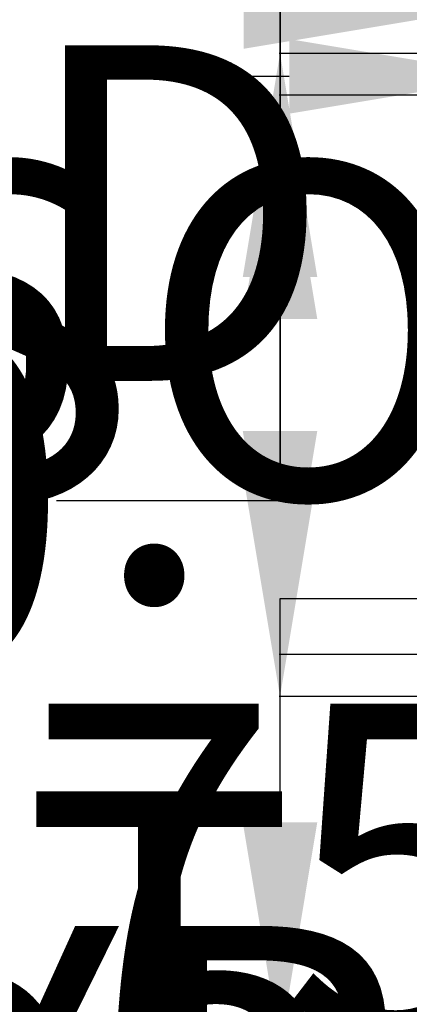
# Model space of a CAD drawing. Units: inches. Extents: x -307 to 2141, y -58 to 895.
# Tile 4 of 28: x 469 to 553, y 100 to 312. Entities that reach past the tile are written whole.
import ezdxf

# ---------------------------------------------------------------- set-up
doc = ezdxf.new("R2010")
doc.units = ezdxf.units.IN
doc.header["$MEASUREMENT"] = 0
doc.layers.add('A-ANNO-DIMS', color=2, linetype='Continuous', lineweight=18)
doc.styles.get("Standard").update_dxf_attribs({"font": 'arial.ttf'})
doc.dimstyles.get("Standard").update_dxf_attribs({"dimtxt": 72, "dimasz": 48, "dimexe": 0.18, "dimexo": 0.0625, "dimgap": 0.09, "dimtad": 0, "dimtih": 1, "dimtoh": 1, "dimdec": 0, "dimrnd": 48, "dimzin": 0, "dimdsep": 46, "dimlunit": 3, "dimtxsty": 'Standard', "dimcen": 0.09, "dimadec": 0, "dimazin": 0, "dimtfac": 1, "dimtdec": 0, "dimtofl": 0, "dimtmove": 0, "dimatfit": 3, "dimfxl": 1, "dimtolj": 1, "dimtzin": 0, "dimarcsym": 0})

# ---------------------------------------------------------------- blocks, each defined once
blk = doc.blocks.new('*D28')
at = {"layer": 'A-ANNO-DIMS', "color": 0, "lineweight": -2, "transparency": 16777216}
for p, q in [((795.36, 433.55), (777.92, 433.55)), ((778.1, 385.55), (778.1, 366.07)), ((795.36, 318.07), (777.92, 318.07)), ((778.1, 318.07), (778.1, 270.07)), ((778.1, 270.07), (730.1, 270.07))]:
    blk.add_line(p, q, dxfattribs=at)
at = {"layer": 'A-ANNO-DIMS', "color": 0, "transparency": 16777216}
for points in [[(770.1, 385.55), (786.1, 385.55), (778.1, 433.55)], [(770.1, 366.07), (786.1, 366.07), (778.1, 318.07)]]:
    blk.add_solid(points, dxfattribs=at)
at = {"layer": 'Defpoints', "color": 0, "transparency": 16777216}
for p in [(795.42, 433.55), (778.1, 318.07), (795.42, 318.07)]:
    blk.add_point(p, dxfattribs=at)
at = {"layer": 'A-ANNO-DIMS', "color": 0, "transparency": 16777216, "insert": (534.42, 270.07), "char_height": 72, "attachment_point": 5}
blk.add_mtext('\\A1;BED 115', dxfattribs=at)
blk = doc.blocks.new('*D36')
at = {"layer": 'A-ANNO-DIMS', "color": 0, "lineweight": -2, "transparency": 16777216}
for p, q in [((871.71, 562.4), (871.76, 610.4)), ((876.55, 514.4), (871.47, 514.4)), ((876.51, 481.35), (871.44, 481.36)), ((871.56, 433.36), (871.51, 385.36)), ((871.51, 385.36), (823.51, 385.36))]:
    blk.add_line(p, q, dxfattribs=at)
at = {"layer": 'A-ANNO-DIMS', "color": 0, "transparency": 16777216}
for points in [[(863.71, 562.41), (879.71, 562.4), (871.65, 514.4)], [(863.56, 433.37), (879.56, 433.35), (871.62, 481.36)]]:
    blk.add_solid(points, dxfattribs=at)
at = {"layer": 'Defpoints', "color": 0, "transparency": 16777216}
for p in [(876.61, 514.4), (871.62, 481.36), (876.57, 481.35)]:
    blk.add_point(p, dxfattribs=at)
at = {"layer": 'A-ANNO-DIMS', "color": 0, "transparency": 16777216, "insert": (548.95, 385.36), "char_height": 72, "attachment_point": 5}
blk.add_mtext('\\A1;WC 33 TYP.', dxfattribs=at)
blk = doc.blocks.new('*D38')
at = {"layer": 'A-ANNO-DIMS', "color": 0, "lineweight": -2, "transparency": 16777216}
for p, q in [((598.5, 222.79), (550.5, 222.79)), ((646.5, 213.85), (646.5, 222.97)), ((706.5, 213.85), (706.5, 222.97)), ((754.5, 222.79), (802.5, 222.79))]:
    blk.add_line(p, q, dxfattribs=at)
at = {"layer": 'A-ANNO-DIMS', "color": 0, "transparency": 16777216}
for points in [[(598.5, 230.79), (598.5, 214.79), (646.5, 222.79)], [(754.5, 230.79), (754.5, 214.79), (706.5, 222.79)]]:
    blk.add_solid(points, dxfattribs=at)
at = {"layer": 'Defpoints', "color": 0, "transparency": 16777216}
for p in [(646.5, 222.79), (646.5, 213.79), (706.5, 213.79)]:
    blk.add_point(p, dxfattribs=at)
at = {"layer": 'A-ANNO-DIMS', "color": 0, "transparency": 16777216, "insert": (97.26, 222.79), "char_height": 72, "attachment_point": 5}
blk.add_mtext('\\A1;LOVESEAT 60 TYP.', dxfattribs=at)
blk = doc.blocks.new('*D39')
at = {"layer": 'A-ANNO-DIMS', "color": 0, "lineweight": -2, "transparency": 16777216}
for p, q in [((637.5, 261.79), (637.5, 309.79)), ((646.43, 213.79), (637.32, 213.79)), ((646.43, 177.12), (637.32, 177.12)), ((637.5, 129.12), (637.5, 81.12)), ((637.5, 81.12), (589.5, 81.12))]:
    blk.add_line(p, q, dxfattribs=at)
at = {"layer": 'A-ANNO-DIMS', "color": 0, "transparency": 16777216}
for points in [[(629.5, 261.79), (645.5, 261.79), (637.5, 213.79)], [(629.5, 129.12), (645.5, 129.12), (637.5, 177.12)]]:
    blk.add_solid(points, dxfattribs=at)
at = {"layer": 'Defpoints', "color": 0, "transparency": 16777216}
for p in [(646.5, 213.79), (637.5, 177.12), (646.5, 177.12)]:
    blk.add_point(p, dxfattribs=at)
at = {"layer": 'A-ANNO-DIMS', "color": 0, "transparency": 16777216, "insert": (414.2, 81.12), "char_height": 72, "attachment_point": 5}
blk.add_mtext('\\A1;37 TYP.', dxfattribs=at)
blk = doc.blocks.new('*D48')
at = {"layer": 'A-ANNO-DIMS', "color": 0, "lineweight": -2, "transparency": 16777216}
for p, q in [((724, 313.98), (724, 361.98)), ((732.94, 265.98), (723.82, 265.98)), ((732.94, 205.98), (723.82, 205.98)), ((724, 157.98), (724, 109.98)), ((724, 109.98), (676, 109.98))]:
    blk.add_line(p, q, dxfattribs=at)
at = {"layer": 'A-ANNO-DIMS', "color": 0, "transparency": 16777216}
for points in [[(716, 313.98), (732, 313.98), (724, 265.98)], [(716, 157.98), (732, 157.98), (724, 205.98)]]:
    blk.add_solid(points, dxfattribs=at)
at = {"layer": 'Defpoints', "color": 0, "transparency": 16777216}
for p in [(733, 265.98), (724, 205.98), (733, 205.98)]:
    blk.add_point(p, dxfattribs=at)
at = {"layer": 'A-ANNO-DIMS', "color": 0, "transparency": 16777216, "insert": (321.56, 109.98), "char_height": 72, "attachment_point": 5}
blk.add_mtext('\\A1;MEDIA UNIT 60', dxfattribs=at)
blk = doc.blocks.new('*D50')
at = {"layer": 'A-ANNO-DIMS', "color": 0, "lineweight": -2, "transparency": 16777216}
for p, q in [((565.34, 315.8), (565.34, 313.15)), ((582.27, 315.8), (582.27, 313.15)), ((517.34, 313.33), (469.34, 313.33)), ((630.27, 313.33), (678.27, 313.33))]:
    blk.add_line(p, q, dxfattribs=at)
at = {"layer": 'A-ANNO-DIMS', "color": 0, "transparency": 16777216}
for points in [[(517.34, 321.33), (517.34, 305.33), (565.34, 313.33)], [(630.27, 321.33), (630.27, 305.33), (582.27, 313.33)]]:
    blk.add_solid(points, dxfattribs=at)
at = {"layer": 'Defpoints', "color": 0, "transparency": 16777216}
for p in [(565.34, 315.87), (582.27, 315.87), (565.34, 313.33)]:
    blk.add_point(p, dxfattribs=at)
at = {"layer": 'A-ANNO-DIMS', "color": 0, "transparency": 16777216, "insert": (226.65, 313.33), "char_height": 72, "attachment_point": 5}
blk.add_mtext('\\A1;PHONE 17', dxfattribs=at)
blk = doc.blocks.new('*D52')
at = {"layer": 'A-ANNO-DIMS', "color": 0, "lineweight": -2, "transparency": 16777216}
for p, q in [((660.21, 554.25), (660.21, 602.25)), ((673.8, 506.25), (660.03, 506.25)), ((673.8, 415.25), (660.03, 415.25)), ((660.21, 367.25), (660.21, 319.25))]:
    blk.add_line(p, q, dxfattribs=at)
at = {"layer": 'A-ANNO-DIMS', "color": 0, "transparency": 16777216}
for points in [[(652.21, 554.25), (668.21, 554.25), (660.21, 506.25)], [(652.21, 367.25), (668.21, 367.25), (660.21, 415.25)]]:
    blk.add_solid(points, dxfattribs=at)
at = {"layer": 'Defpoints', "color": 0, "transparency": 16777216}
for p in [(673.86, 506.25), (660.21, 415.25), (673.86, 415.25)]:
    blk.add_point(p, dxfattribs=at)
at = {"layer": 'A-ANNO-DIMS', "color": 0, "transparency": 16777216, "insert": (660.21, 460.75), "char_height": 72, "attachment_point": 5}
blk.add_mtext('\\A1;DINING SET 91', dxfattribs=at)
blk = doc.blocks.new('*D58')
at = {"layer": 'A-ANNO-DIMS', "color": 0, "lineweight": -2, "transparency": 16777216}
for p, q in [((624.38, 334.8), (624.38, 382.8)), ((611.84, 286.8), (624.56, 286.8)), ((611.84, 202.8), (624.56, 202.8)), ((624.38, 154.8), (624.38, 106.8))]:
    blk.add_line(p, q, dxfattribs=at)
at = {"layer": 'A-ANNO-DIMS', "color": 0, "transparency": 16777216}
for points in [[(616.38, 334.8), (632.38, 334.8), (624.38, 286.8)], [(616.38, 154.8), (632.38, 154.8), (624.38, 202.8)]]:
    blk.add_solid(points, dxfattribs=at)
at = {"layer": 'Defpoints', "color": 0, "transparency": 16777216}
for p in [(611.78, 286.8), (624.38, 286.8), (611.78, 202.8)]:
    blk.add_point(p, dxfattribs=at)
at = {"layer": 'A-ANNO-DIMS', "color": 0, "transparency": 16777216, "insert": (624.38, 244.8), "char_height": 72, "attachment_point": 5}
blk.add_mtext('\\A1;SOFA 84', dxfattribs=at)
blk = doc.blocks.new('*D59')
at = {"layer": 'A-ANNO-DIMS', "color": 0, "lineweight": -2, "transparency": 16777216}
for p, q in [((527.11, 299.4), (479.11, 299.4)), ((575.11, 286.86), (575.11, 299.58)), ((611.78, 286.86), (611.78, 299.58)), ((659.78, 299.4), (707.78, 299.4))]:
    blk.add_line(p, q, dxfattribs=at)
at = {"layer": 'A-ANNO-DIMS', "color": 0, "transparency": 16777216}
for points in [[(527.11, 307.4), (527.11, 291.4), (575.11, 299.4)], [(659.78, 307.4), (659.78, 291.4), (611.78, 299.4)]]:
    blk.add_solid(points, dxfattribs=at)
at = {"layer": 'Defpoints', "color": 0, "transparency": 16777216}
for p in [(575.11, 299.4), (575.11, 286.8), (611.78, 286.8)]:
    blk.add_point(p, dxfattribs=at)
at = {"layer": 'A-ANNO-DIMS', "color": 0, "transparency": 16777216, "insert": (427.48, 299.4), "char_height": 72, "attachment_point": 5}
blk.add_mtext('\\A1;37', dxfattribs=at)
blk = doc.blocks.new('*D64')
at = {"layer": 'A-ANNO-DIMS', "color": 0, "lineweight": -2, "transparency": 16777216}
for p, q in [((556.27, 691.34), (524.95, 691.34)), ((525.13, 643.34), (525.13, 465.69)), ((525.13, 214.34), (525.13, 391.99)), ((556.27, 166.34), (524.95, 166.34))]:
    blk.add_line(p, q, dxfattribs=at)
at = {"layer": 'A-ANNO-DIMS', "color": 0, "transparency": 16777216}
for points in [[(517.13, 643.34), (533.13, 643.34), (525.13, 691.34)], [(517.13, 214.34), (533.13, 214.34), (525.13, 166.34)]]:
    blk.add_solid(points, dxfattribs=at)
at = {"layer": 'Defpoints', "color": 0, "transparency": 16777216}
for p in [(525.13, 691.34), (556.34, 691.34), (556.34, 166.34)]:
    blk.add_point(p, dxfattribs=at)
at = {"layer": 'A-ANNO-DIMS', "color": 0, "transparency": 16777216, "insert": (525.13, 428.84), "char_height": 72, "attachment_point": 5}
blk.add_mtext('\\A1;525', dxfattribs=at)
blk = doc.blocks.new('*D65')
at = {"layer": 'A-ANNO-DIMS', "color": 0, "lineweight": -2, "transparency": 16777216}
for p, q in [((587.54, 252.57), (587.54, 300.57)), ((556.4, 204.57), (587.72, 204.57)), ((556.4, 166.34), (587.72, 166.34)), ((587.54, 118.34), (587.54, 70.34)), ((587.54, 70.34), (539.54, 70.34))]:
    blk.add_line(p, q, dxfattribs=at)
at = {"layer": 'A-ANNO-DIMS', "color": 0, "transparency": 16777216}
for points in [[(579.54, 252.57), (595.54, 252.57), (587.54, 204.57)], [(579.54, 118.34), (595.54, 118.34), (587.54, 166.34)]]:
    blk.add_solid(points, dxfattribs=at)
at = {"layer": 'Defpoints', "color": 0, "transparency": 16777216}
for p in [(556.34, 204.57), (556.34, 166.34), (587.54, 166.34)]:
    blk.add_point(p, dxfattribs=at)
at = {"layer": 'A-ANNO-DIMS', "color": 0, "transparency": 16777216, "insert": (417.99, 70.34), "char_height": 72, "attachment_point": 5}
blk.add_mtext('\\A1;38.23', dxfattribs=at)
blk = doc.blocks.new('*D66')
at = {"layer": 'A-ANNO-DIMS', "color": 0, "lineweight": -2, "transparency": 16777216}
for p, q in [((525.13, 382.34), (525.13, 430.34)), ((556.27, 334.34), (524.95, 334.34)), ((565.27, 304.34), (524.95, 304.34)), ((525.13, 256.34), (525.13, 208.34)), ((525.13, 208.34), (477.13, 208.34))]:
    blk.add_line(p, q, dxfattribs=at)
at = {"layer": 'A-ANNO-DIMS', "color": 0, "transparency": 16777216}
for points in [[(517.13, 382.34), (533.13, 382.34), (525.13, 334.34)], [(517.13, 256.34), (533.13, 256.34), (525.13, 304.34)]]:
    blk.add_solid(points, dxfattribs=at)
at = {"layer": 'Defpoints', "color": 0, "transparency": 16777216}
for p in [(556.34, 334.34), (525.13, 304.34), (565.34, 304.34)]:
    blk.add_point(p, dxfattribs=at)
at = {"layer": 'A-ANNO-DIMS', "color": 0, "transparency": 16777216, "insert": (425.62, 208.34), "char_height": 72, "attachment_point": 5}
blk.add_mtext('\\A1;30', dxfattribs=at)
blk = doc.blocks.new('*D67')
at = {"layer": 'A-ANNO-DIMS', "color": 0, "lineweight": -2, "transparency": 16777216}
for p, q in [((525.13, 496.83), (525.13, 544.83)), ((556.27, 448.83), (524.95, 448.83)), ((556.27, 370.34), (524.95, 370.34)), ((525.13, 322.34), (525.13, 274.34))]:
    blk.add_line(p, q, dxfattribs=at)
at = {"layer": 'A-ANNO-DIMS', "color": 0, "transparency": 16777216}
for points in [[(517.13, 496.83), (533.13, 496.83), (525.13, 448.83)], [(517.13, 322.34), (533.13, 322.34), (525.13, 370.34)]]:
    blk.add_solid(points, dxfattribs=at)
at = {"layer": 'Defpoints', "color": 0, "transparency": 16777216}
for p in [(525.13, 448.83), (556.34, 448.83), (556.34, 370.34)]:
    blk.add_point(p, dxfattribs=at)
at = {"layer": 'A-ANNO-DIMS', "color": 0, "transparency": 16777216, "insert": (525.13, 409.59), "char_height": 72, "attachment_point": 5}
blk.add_mtext('\\A1;78.49', dxfattribs=at)
blk = doc.blocks.new('*D70')
at = {"layer": 'A-ANNO-DIMS', "color": 0, "lineweight": -2, "transparency": 16777216}
for p, q in [((525.13184, 214.340828), (525.13184, 262.340828)), ((556.27334, 166.340828), (524.95184, 166.340828)), ((556.27334, 91.340828), (524.95184, 91.340828)), ((525.13184, 43.340828), (525.13184, -4.659172))]:
    blk.add_line(p, q, dxfattribs=at)
at = {"layer": 'A-ANNO-DIMS', "color": 0, "transparency": 16777216}
for points in [[(517.13184, 214.340828), (533.13184, 214.340828), (525.13184, 166.340828)], [(517.13184, 43.340828), (533.13184, 43.340828), (525.13184, 91.340828)]]:
    blk.add_solid(points, dxfattribs=at)
at = {"layer": 'Defpoints', "color": 0, "transparency": 16777216}
for p in [(525.13184, 166.340828), (556.33584, 166.340828), (556.33584, 91.340828)]:
    blk.add_point(p, dxfattribs=at)
at = {"layer": 'A-ANNO-DIMS', "color": 0, "transparency": 16777216, "insert": (525.13184, 128.840828), "char_height": 72, "attachment_point": 5}
blk.add_mtext('\\A1;75', dxfattribs=at)
blk = doc.blocks.new('*D71')
at = {"layer": 'A-ANNO-DIMS', "color": 0, "lineweight": -2, "transparency": 16777216}
for p, q in [((525.13, 139.34), (525.13, 187.34)), ((525.13, 187.34), (573.13, 187.34)), ((632.56, 91.34), (524.95, 91.34)), ((632.56, 67.34), (524.95, 67.34)), ((525.13, 19.34), (525.13, -28.66))]:
    blk.add_line(p, q, dxfattribs=at)
at = {"layer": 'A-ANNO-DIMS', "color": 0, "transparency": 16777216}
for points in [[(517.13, 139.34), (533.13, 139.34), (525.13, 91.34)], [(517.13, 19.34), (533.13, 19.34), (525.13, 67.34)]]:
    blk.add_solid(points, dxfattribs=at)
at = {"layer": 'Defpoints', "color": 0, "transparency": 16777216}
for p in [(525.13, 91.34), (632.62, 91.34), (632.62, 67.34)]:
    blk.add_point(p, dxfattribs=at)
at = {"layer": 'A-ANNO-DIMS', "color": 0, "transparency": 16777216, "insert": (625.26, 187.34), "char_height": 72, "attachment_point": 5}
blk.add_mtext('\\A1;24', dxfattribs=at)
blk = doc.blocks.new('*D86')
at = {"layer": 'A-ANNO-DIMS', "color": 0, "lineweight": -2, "transparency": 16777216}
for p, q in [((565.34, 304.28), (565.34, 35.96)), ((625.34, 304.28), (625.34, 35.96)), ((517.34, 36.14), (469.34, 36.14)), ((673.34, 36.14), (721.34, 36.14))]:
    blk.add_line(p, q, dxfattribs=at)
at = {"layer": 'A-ANNO-DIMS', "color": 0, "transparency": 16777216}
for points in [[(517.34, 44.14), (517.34, 28.14), (565.34, 36.14)], [(673.34, 44.14), (673.34, 28.14), (625.34, 36.14)]]:
    blk.add_solid(points, dxfattribs=at)
at = {"layer": 'Defpoints', "color": 0, "transparency": 16777216}
for p in [(565.34, 304.34), (625.34, 304.34), (625.34, 36.14)]:
    blk.add_point(p, dxfattribs=at)
at = {"layer": 'A-ANNO-DIMS', "color": 0, "transparency": 16777216, "insert": (773.07, 36.14), "char_height": 72, "attachment_point": 5}
blk.add_mtext('\\A1;60', dxfattribs=at)
blk = doc.blocks.new('*D87')
at = {"layer": 'A-ANNO-DIMS', "color": 0, "lineweight": -2, "transparency": 16777216}
for p, q in [((525.13184, 448.340828), (525.13184, 496.340828)), ((625.27334, 400.340828), (524.95184, 400.340828)), ((625.27334, 304.340828), (524.95184, 304.340828)), ((525.13184, 256.340828), (525.13184, 208.340828))]:
    blk.add_line(p, q, dxfattribs=at)
at = {"layer": 'A-ANNO-DIMS', "color": 0, "transparency": 16777216}
for points in [[(517.13184, 448.340828), (533.13184, 448.340828), (525.13184, 400.340828)], [(517.13184, 256.340828), (533.13184, 256.340828), (525.13184, 304.340828)]]:
    blk.add_solid(points, dxfattribs=at)
at = {"layer": 'Defpoints', "color": 0, "transparency": 16777216}
for p in [(525.13184, 400.340828), (625.33584, 400.340828), (625.33584, 304.340828)]:
    blk.add_point(p, dxfattribs=at)
at = {"layer": 'A-ANNO-DIMS', "color": 0, "transparency": 16777216, "insert": (525.13184, 352.340828), "char_height": 72, "attachment_point": 5}
blk.add_mtext('\\A1;96', dxfattribs=at)
blk = doc.blocks.new('*D88')
at = {"layer": 'A-ANNO-DIMS', "color": 0, "lineweight": -2, "transparency": 16777216}
for p, q in [((517.33584, 722.544828), (469.33584, 722.544828)), ((565.33584, 295.403328), (565.33584, 722.724828)), ((754.33584, 271.403328), (754.33584, 722.724828)), ((802.33584, 722.544828), (850.33584, 722.544828))]:
    blk.add_line(p, q, dxfattribs=at)
at = {"layer": 'A-ANNO-DIMS', "color": 0, "transparency": 16777216}
for points in [[(517.33584, 730.544828), (517.33584, 714.544828), (565.33584, 722.544828)], [(802.33584, 730.544828), (802.33584, 714.544828), (754.33584, 722.544828)]]:
    blk.add_solid(points, dxfattribs=at)
at = {"layer": 'Defpoints', "color": 0, "transparency": 16777216}
for p in [(754.33584, 722.544828), (565.33584, 295.340828), (754.33584, 271.340828)]:
    blk.add_point(p, dxfattribs=at)
at = {"layer": 'A-ANNO-DIMS', "color": 0, "transparency": 16777216, "insert": (659.83584, 722.544828), "char_height": 72, "attachment_point": 5}
blk.add_mtext('\\A1;189', dxfattribs=at)
blk = doc.blocks.new('*D89')
at = {"layer": 'A-ANNO-DIMS', "color": 0, "lineweight": -2, "transparency": 16777216}
for p, q in [((525.13, 295.34), (525.13, 343.34)), ((525.13, 343.34), (573.13, 343.34)), ((565.27, 295.34), (524.95, 295.34)), ((525.13, 223.34), (525.13, 247.34)), ((556.27, 175.34), (524.95, 175.34))]:
    blk.add_line(p, q, dxfattribs=at)
at = {"layer": 'A-ANNO-DIMS', "color": 0, "transparency": 16777216}
for points in [[(517.13, 247.34), (533.13, 247.34), (525.13, 295.34)], [(517.13, 223.34), (533.13, 223.34), (525.13, 175.34)]]:
    blk.add_solid(points, dxfattribs=at)
at = {"layer": 'Defpoints', "color": 0, "transparency": 16777216}
for p in [(525.13, 295.34), (565.34, 295.34), (556.34, 175.34)]:
    blk.add_point(p, dxfattribs=at)
at = {"layer": 'A-ANNO-DIMS', "color": 0, "transparency": 16777216, "insert": (649.25, 343.34), "char_height": 72, "attachment_point": 5}
blk.add_mtext('\\A1;120', dxfattribs=at)
blk = doc.blocks.new('*D90')
at = {"layer": 'A-ANNO-DIMS', "color": 0, "lineweight": -2, "transparency": 16777216}
for p, q in [((556.34, 166.28), (556.34, 35.96)), ((589.34, 166.28), (589.34, 35.96)), ((508.34, 36.14), (460.34, 36.14)), ((637.34, 36.14), (685.34, 36.14))]:
    blk.add_line(p, q, dxfattribs=at)
at = {"layer": 'A-ANNO-DIMS', "color": 0, "transparency": 16777216}
for points in [[(508.34, 44.14), (508.34, 28.14), (556.34, 36.14)], [(637.34, 44.14), (637.34, 28.14), (589.34, 36.14)]]:
    blk.add_solid(points, dxfattribs=at)
at = {"layer": 'Defpoints', "color": 0, "transparency": 16777216}
for p in [(556.34, 166.34), (589.34, 166.34), (589.34, 36.14)]:
    blk.add_point(p, dxfattribs=at)
at = {"layer": 'A-ANNO-DIMS', "color": 0, "transparency": 16777216, "insert": (736.97, 36.14), "char_height": 72, "attachment_point": 5}
blk.add_mtext('\\A1;33', dxfattribs=at)
blk = doc.blocks.new('*D91')
at = {"layer": 'A-ANNO-DIMS', "color": 0, "lineweight": -2, "transparency": 16777216}
for p, q in [((589.34, 166.28), (589.34, 35.96)), ((637.34, 166.28), (637.34, 35.96)), ((541.34, 36.14), (493.34, 36.14)), ((685.34, 36.14), (733.34, 36.14))]:
    blk.add_line(p, q, dxfattribs=at)
at = {"layer": 'A-ANNO-DIMS', "color": 0, "transparency": 16777216}
for points in [[(541.34, 44.14), (541.34, 28.14), (589.34, 36.14)], [(685.34, 44.14), (685.34, 28.14), (637.34, 36.14)]]:
    blk.add_solid(points, dxfattribs=at)
at = {"layer": 'Defpoints', "color": 0, "transparency": 16777216}
for p in [(589.34, 166.34), (637.34, 166.34), (637.34, 36.14)]:
    blk.add_point(p, dxfattribs=at)
at = {"layer": 'A-ANNO-DIMS', "color": 0, "transparency": 16777216, "insert": (786.52, 36.14), "char_height": 72, "attachment_point": 5}
blk.add_mtext('\\A1;48', dxfattribs=at)
blk = doc.blocks.new('*D92')
at = {"layer": 'A-ANNO-DIMS', "color": 0, "lineweight": -2, "transparency": 16777216}
for p, q in [((637.34, 166.28), (637.34, 35.96)), ((664.34, 166.28), (664.34, 35.96)), ((589.34, 36.14), (541.34, 36.14)), ((712.34, 36.14), (760.34, 36.14))]:
    blk.add_line(p, q, dxfattribs=at)
at = {"layer": 'A-ANNO-DIMS', "color": 0, "transparency": 16777216}
for points in [[(589.34, 44.14), (589.34, 28.14), (637.34, 36.14)], [(712.34, 44.14), (712.34, 28.14), (664.34, 36.14)]]:
    blk.add_solid(points, dxfattribs=at)
at = {"layer": 'Defpoints', "color": 0, "transparency": 16777216}
for p in [(637.34, 166.34), (664.34, 166.34), (664.34, 36.14)]:
    blk.add_point(p, dxfattribs=at)
at = {"layer": 'A-ANNO-DIMS', "color": 0, "transparency": 16777216, "insert": (812.61, 36.14), "char_height": 72, "attachment_point": 5}
blk.add_mtext('\\A1;27', dxfattribs=at)
blk = doc.blocks.new('*D100')
at = {"layer": 'A-ANNO-DIMS', "color": 0, "lineweight": -2, "transparency": 16777216}
for p, q in [((589.34, 409.28), (589.34, 35.96)), ((625.34, 409.28), (625.34, 35.96)), ((541.34, 36.14), (493.34, 36.14)), ((673.34, 36.14), (721.34, 36.14))]:
    blk.add_line(p, q, dxfattribs=at)
at = {"layer": 'A-ANNO-DIMS', "color": 0, "transparency": 16777216}
for points in [[(541.34, 44.14), (541.34, 28.14), (589.34, 36.14)], [(673.34, 44.14), (673.34, 28.14), (625.34, 36.14)]]:
    blk.add_solid(points, dxfattribs=at)
at = {"layer": 'Defpoints', "color": 0, "transparency": 16777216}
for p in [(589.34, 409.34), (625.34, 409.34), (625.34, 36.14)]:
    blk.add_point(p, dxfattribs=at)
at = {"layer": 'A-ANNO-DIMS', "color": 0, "transparency": 16777216, "insert": (772.95, 36.14), "char_height": 72, "attachment_point": 5}
blk.add_mtext('\\A1;36', dxfattribs=at)

msp = doc.modelspace()

# ---------------------------------------------------------------- dimensions: what is measured, and where the dimension line sits
at = {"layer": 'A-ANNO-DIMS'}
for base, p1, p2, picture, middle in [((754.3358, 722.5448), (565.3358, 295.3408), (754.3358, 271.3408), '*D88', (659.8358, 722.5448)), ((625.3358, 36.1368), (589.339, 409.3408), (625.3358, 409.3408), '*D100', (772.9456, 36.1368)), ((625.3358, 36.1368), (565.3358, 304.3408), (625.3358, 304.3408), '*D86', (773.0684, 36.1368)), ((589.3358, 36.1368), (556.3358, 166.3408), (589.3358, 166.3408), '*D90', (736.9702, 36.1368)), ((637.3358, 36.1368), (589.3358, 166.3408), (637.3358, 166.3408), '*D91', (786.5172, 36.1368)), ((664.3358, 36.1368), (637.3358, 166.3408), (664.3358, 166.3408), '*D92', (812.6087, 36.1368))]:
    dim = msp.add_linear_dim(base=base, p1=p1, p2=p2, dimstyle='Standard', override={"dimdec": 0, "dimlfac": 1, "dimrnd": 0, "dimzin": 0, "dimdsep": 46, "dimlunit": 2}, dxfattribs=at)
    dim.commit()
    dim.dimension.update_dxf_attribs({"geometry": picture, "text_midpoint": middle})
for base, p1, p2, angle, override, picture, middle in [((525.1318, 691.3408), (556.3358, 166.3408), (556.3358, 691.3408), 90, {"dimdec": 0, "dimlfac": 1, "dimrnd": 0, "dimzin": 0, "dimdsep": 46, "dimlunit": 2}, '*D64', (525.1318, 428.8408)), ((525.1318, 448.8333), (556.3358, 370.3416), (556.3358, 448.8333), 90, {"dimdec": 2, "dimlfac": 1, "dimrnd": 0, "dimzin": 0, "dimdsep": 46, "dimlunit": 2}, '*D67', (525.1318, 409.5874)), ((525.1318, 400.3408), (625.3358, 304.3408), (625.3358, 400.3408), 90, {"dimdec": 0, "dimlfac": 1, "dimrnd": 0, "dimzin": 0, "dimdsep": 46, "dimlunit": 2}, '*D87', (525.1318, 352.3408)), ((525.1318, 304.3408), (556.3358, 334.3416), (565.3358, 304.3408), 90, {"dimdec": 0, "dimlfac": 1, "dimrnd": 0, "dimzin": 0, "dimdsep": 46, "dimlunit": 2}, '*D66', (425.6203, 208.3408)), ((525.1318, 295.3408), (556.3358, 175.3408), (565.3358, 295.3408), 90, {"dimdec": 0, "dimlfac": 1, "dimrnd": 0, "dimzin": 0, "dimdsep": 46, "dimlunit": 2}, '*D89', (649.2491, 343.3408)), ((575.1104, 299.3976), (611.777, 286.7976), (575.1104, 286.7976), 180, {"dimdec": 0, "dimlfac": 1, "dimrnd": 0, "dimzin": 0, "dimdsep": 46, "dimlunit": 2}, '*D59', (427.476, 299.3976)), ((587.5398, 166.3408), (556.3358, 204.574), (556.3358, 166.3408), 270, {"dimdec": 2, "dimlfac": 1, "dimrnd": 0, "dimzin": 0, "dimdsep": 46, "dimlunit": 2}, '*D65', (417.9928, 70.3408)), ((525.1318, 166.3408), (556.3358, 91.3408), (556.3358, 166.3408), 90, {"dimdec": 0, "dimlfac": 1, "dimrnd": 0, "dimzin": 0, "dimdsep": 46, "dimlunit": 2}, '*D70', (525.1318, 128.8408)), ((525.1318, 91.3408), (632.6211, 67.3408), (632.6211, 91.3408), 90, {"dimdec": 0, "dimlfac": 1, "dimrnd": 0, "dimzin": 0, "dimdsep": 46, "dimlunit": 2}, '*D71', (625.2573, 187.3408))]:
    dim = msp.add_linear_dim(base=base, p1=p1, p2=p2, angle=angle, dimstyle='Standard', override=override, dxfattribs=at)
    dim.commit()
    dim.dimension.update_dxf_attribs({"geometry": picture, "text_midpoint": middle})
for base, p1, p2, angle, text, picture, middle in [((660.2083, 415.2485), (673.8583, 506.2485), (673.8583, 415.2485), 270, 'DINING SET <>', '*D52', (660.2083, 460.7485)), ((871.6167, 481.3581), (876.6106, 514.3988), (876.5736, 481.3526), 269.935892, 'WC <> TYP.', '*D36', (548.95, 385.3582)), ((778.0993, 318.073), (795.4208, 433.5496), (795.4208, 318.073), 270, 'BED <>', '*D28', (534.4158, 270.073)), ((565.3358, 313.3263), (582.2714, 315.8666), (565.3358, 315.8666), 180, 'PHONE <>', '*D50', (226.651, 313.3263)), ((646.4965, 222.7908), (706.4965, 213.7908), (646.4965, 213.7908), 180, 'LOVESEAT <> TYP.', '*D38', (97.2632, 222.7908)), ((624.377, 286.7976), (611.777, 202.7976), (611.777, 286.7976), 90, 'SOFA <>', '*D58', (624.377, 244.7976)), ((724.0025, 205.9815), (733.0025, 265.9815), (733.0025, 205.9815), 270, 'MEDIA UNIT <>', '*D48', (321.5605, 109.9815)), ((637.4965, 177.1242), (646.4965, 213.7908), (646.4965, 177.1242), 270, '<> TYP.', '*D39', (414.195, 81.1242))]:
    dim = msp.add_linear_dim(base=base, p1=p1, p2=p2, angle=angle, text=text, dimstyle='Standard', override={"dimdec": 0, "dimlfac": 1, "dimrnd": 0, "dimzin": 0, "dimdsep": 46, "dimlunit": 2}, dxfattribs=at)
    dim.commit()
    dim.dimension.update_dxf_attribs({"geometry": picture, "text_midpoint": middle})

doc.saveas('drawing.dxf')
